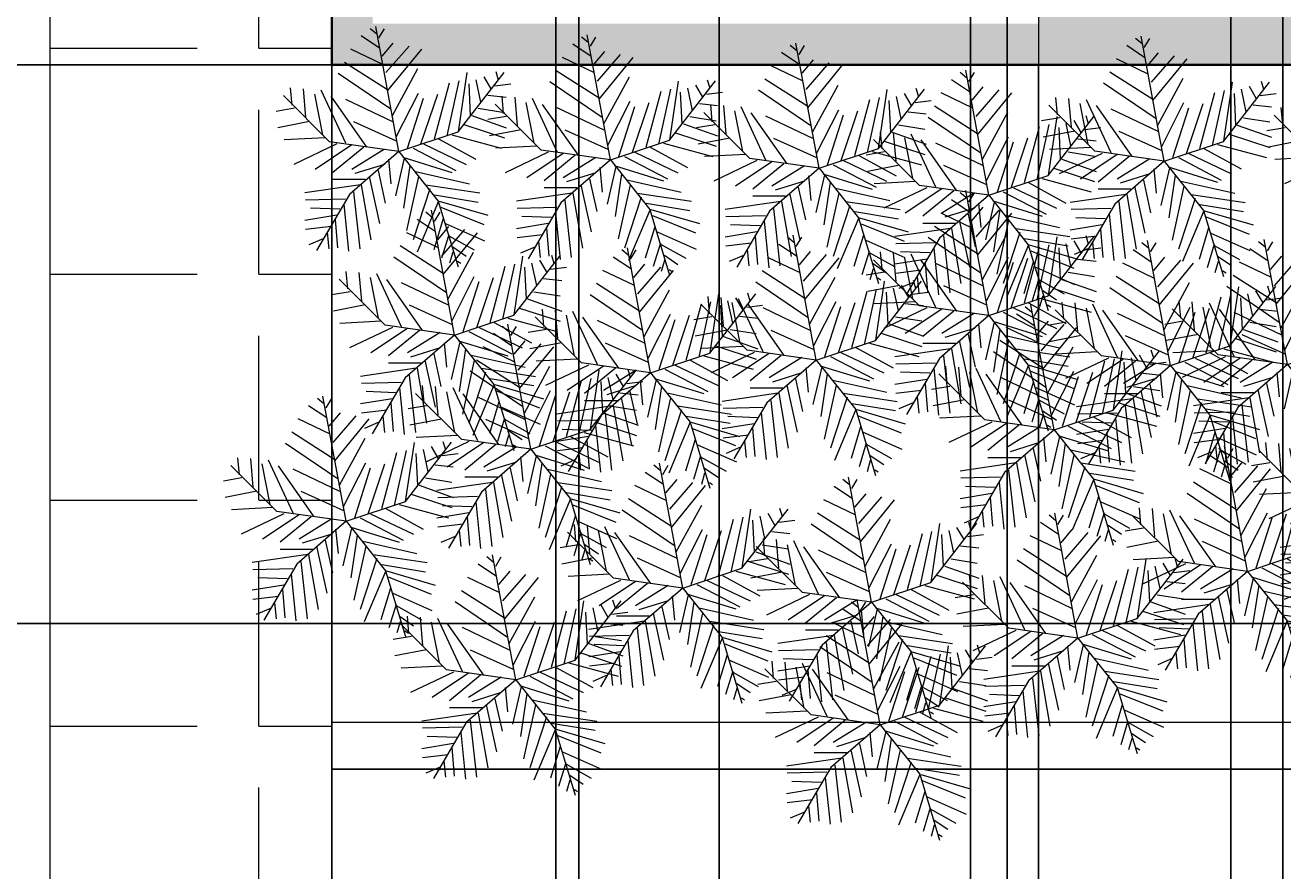
# Model space of a CAD drawing. Units: inches. Extents: x 818 to 1898, y 976 to 2364.
# Tile 20 of 96: x 1405 to 1512, y 1277 to 1349. Entities that reach past the tile are written whole.
import ezdxf

# ---------------------------------------------------------------- set-up
doc = ezdxf.new("R2010")
doc.units = ezdxf.units.IN
doc.header["$LTSCALE"] = 5
doc.header["$MEASUREMENT"] = 0
for name, color, linetype, lineweight in [('A-ANNO-DIMS', 2, 'Continuous', 18), ('A-GLAZ', 4, 'Continuous', 18), ('A-WALL', 7, 'Continuous', 40), ('C-PKNG', 8, 'Continuous', 18), ('C-PKNG-PATT', 9, 'Continuous', 9), ('L-PLNT-BEDS', 94, 'Continuous', 18)]:
    doc.layers.add(name, color=color, linetype=linetype, lineweight=lineweight)
for name, color, linetype, lineweight, true_color in [('A-GLAZ-PATT', 141, 'Continuous', 9, 0xadddf7), ('A-WALL-PATT', 251, 'Continuous', 13, 0x636466), ('L-PLNT', 116, 'Continuous', 13, 0x136734)]:
    doc.layers.add(name, color=color, linetype=linetype, lineweight=lineweight, true_color=true_color)
doc.styles.get("Standard").update_dxf_attribs({"font": 'arial.ttf'})
doc.dimstyles.get("Standard").update_dxf_attribs({"dimtxt": 0.18, "dimasz": 0.18, "dimexe": 0.18, "dimexo": 0.0625, "dimgap": 0.09, "dimtad": 0, "dimtih": 1, "dimtoh": 1, "dimdec": 4, "dimzin": 0, "dimdsep": 46, "dimtxsty": 'Standard', "dimcen": 0.09, "dimadec": 0, "dimazin": 0, "dimtfac": 1, "dimtdec": 4, "dimtofl": 0, "dimtmove": 0, "dimatfit": 3, "dimfxl": 1, "dimtolj": 1, "dimtzin": 0, "dimarcsym": 0})
pattern_1 = [(0, (0, 0), (0, 19.25), [14, -5.25]), (90, (0, 0), (-19.25, 1e-15), [14, -5.25])]

# ---------------------------------------------------------------- blocks, each defined once
blk = doc.blocks.new('SHRUB-ACCENT')
for p, q in [((10.44, 9.82), (8.47, 20.47)), ((8.8, 18.63), (7.25, 19.67)), ((8.53, 19.84), (7.99, 20.28)), ((8.74, 19.5), (9.21, 20.28)), ((9.08, 17.24), (6.37, 18.54)), ((9.01, 17.93), (9.96, 19.06)), ((9.35, 16.54), (11.31, 18.8)), ((9.48, 14.98), (12.39, 18.54)), ((9.48, 15.07), (5.82, 17.41)), ((9.75, 13.42), (5.28, 16.46)), ((9.89, 12.9), (12.06, 16.89)), ((15.49, 11.5), (19.41, 16.55)), ((15.51, 11.51), (16.25, 16.54)), ((17.68, 16.2), (18.29, 15.16)), ((18.69, 16.63), (18.9, 15.94)), ((1.35, 13.77), (1.22, 15.24)), ((2.3, 15.16), (2.51, 12.72)), ((3.79, 15.07), (5.89, 10.55)), ((13.48, 10.9), (14.76, 15.68)), ((14.56, 11.16), (15.58, 15.85)), ((16.39, 15.59), (16.53, 12.9)), ((17, 15.94), (17.41, 14.03)), ((18.62, 15.42), (19.98, 15.59)), ((4.55, 10.66), (0.62, 14.58)), ((3.25, 14.72), (3.93, 11.25)), ((7.72, 10.21), (4.67, 14.55)), ((5.89, 14.29), (9.89, 12.38)), ((10.23, 11.07), (12.12, 14.81)), ((11.17, 10.12), (12.53, 14.37)), ((12.33, 10.47), (13.75, 14.72)), ((18.02, 14.63), (19.57, 14.46)), ((1.56, 13.51), (0, 13.25)), ((16.66, 12.9), (19.57, 11.86)), ((17.2, 13.51), (19.44, 13.16)), ((2.84, 12.38), (0.14, 11.86)), ((6.57, 12.38), (10.23, 10.73)), ((15.98, 12.12), (19.44, 10.99)), ((4.2, 10.99), (0.68, 10.81)), ((10.44, 9.82), (15.49, 11.5)), ((13.82, 10.9), (17, 9.16)), ((14.97, 11.25), (19.17, 10.12)), ((5.15, 10.47), (1.49, 8.73)), ((6.43, 10.38), (3.32, 8.3)), ((10.44, 9.82), (4.55, 10.66)), ((7.45, 10.21), (4.81, 8.04)), ((10.44, 9.82), (6.23, 6.17)), ((9.21, 10.03), (6.43, 8.3)), ((10.44, 9.82), (13.8, 5.61)), ((11.65, 10.12), (15.31, 8.21)), ((12.53, 10.47), (16.19, 8.73)), ((9.21, 8.73), (6.7, 7.95)), ((9.55, 9.16), (9.75, 7.08)), ((10.9, 9.25), (10.16, 6.04)), ((10.77, 9.34), (14.97, 8.04)), ((11.38, 8.64), (10.84, 5)), ((7.92, 7.69), (8.8, 3.69)), ((8.67, 8.21), (9.28, 5.43)), ((12.12, 7.69), (11.11, 3.09)), ((11.85, 8.12), (16.46, 7.08)), ((7.18, 6.99), (2.44, 6.3)), ((7.59, 7.43), (4.81, 7.43)), ((7.25, 6.99), (8.06, 2.31)), ((13.07, 6.65), (11.65, 2.31)), ((12.73, 6.99), (17.34, 6.3)), ((5.89, 5.78), (2.51, 5.69)), ((6.23, 6.17), (3.43, 1.4)), ((6.57, 6.39), (7.11, 1.52)), ((13.82, 5.6), (11.99, 1.26)), ((13.48, 6.13), (17.2, 5.52)), ((13.8, 5.61), (15.49, 0)), ((13.88, 5.6), (18.02, 4.39)), ((5.15, 4.39), (2.44, 3.95)), ((5.42, 4.91), (2.91, 5)), ((5.76, 5.34), (6.16, 1.35)), ((14.02, 5.08), (17.68, 3.61)), ((4.67, 3.43), (2.51, 3.17)), ((5.01, 4.04), (5.21, 1.61)), ((14.22, 4.13), (13.41, 1.44)), ((14.43, 3.69), (17.74, 2.22)), ((4, 2.39), (2.78, 1.87)), ((4.33, 2.91), (4.47, 1.52)), ((14.7, 2.74), (14.09, 0.74)), ((14.7, 2.65), (16.86, 1.44)), ((15.04, 1.26), (14.76, 0.31)), ((15.04, 1.7), (16.19, 0.92)), ((15.44, 0.48), (15.71, 0.31))]:
    blk.add_line(p, q)
blk = doc.blocks.new('*D61')
at = {"layer": 'A-ANNO-DIMS', "color": 0, "lineweight": -2, "ltscale": 5, "transparency": 16777216}
for p, q in [((1071.73, 1203.03), (1071.73, 2363.87)), ((1430.73, 1203.03), (1430.73, 2363.87)), ((1071.91, 2363.69), (1250.94, 2363.69)), ((1430.55, 2363.69), (1251.51, 2363.69))]:
    blk.add_line(p, q, dxfattribs=at)
at = {"layer": 'A-ANNO-DIMS', "color": 0, "ltscale": 5, "transparency": 16777216}
for points in [[(1071.91, 2363.72), (1071.91, 2363.66), (1071.73, 2363.69)], [(1430.55, 2363.72), (1430.55, 2363.66), (1430.73, 2363.69)]]:
    blk.add_solid(points, dxfattribs=at)
at = {"layer": 'Defpoints', "color": 0, "ltscale": 5, "transparency": 16777216}
for p in [(1430.73, 2363.69), (1071.73, 1202.96), (1430.73, 1202.96)]:
    blk.add_point(p, dxfattribs=at)
at = {"layer": 'A-ANNO-DIMS', "color": 0, "ltscale": 5, "transparency": 16777216, "insert": (1251.23, 2363.69), "char_height": 0.18, "attachment_point": 5}
blk.add_mtext('\\A1;359', dxfattribs=at)
blk = doc.blocks.new('*D65')
at = {"layer": 'A-ANNO-DIMS', "color": 0, "lineweight": -2, "ltscale": 5, "transparency": 16777216}
for p, q in [((1430.73, 1346.02), (1430.73, 975.66)), ((1714.73, 1346.02), (1714.73, 975.66)), ((1430.91, 975.84), (1572.44, 975.84)), ((1714.55, 975.84), (1573.02, 975.84))]:
    blk.add_line(p, q, dxfattribs=at)
at = {"layer": 'A-ANNO-DIMS', "color": 0, "ltscale": 5, "transparency": 16777216}
for points in [[(1430.91, 975.87), (1430.91, 975.81), (1430.73, 975.84)], [(1714.55, 975.87), (1714.55, 975.81), (1714.73, 975.84)]]:
    blk.add_solid(points, dxfattribs=at)
at = {"layer": 'Defpoints', "color": 0, "ltscale": 5, "transparency": 16777216}
for p in [(1430.73, 1346.08), (1714.73, 1346.08), (1714.73, 975.84)]:
    blk.add_point(p, dxfattribs=at)
at = {"layer": 'A-ANNO-DIMS', "color": 0, "ltscale": 5, "transparency": 16777216, "insert": (1572.73, 975.84), "char_height": 0.18, "attachment_point": 5}
blk.add_mtext('\\A1;284', dxfattribs=at)
blk = doc.blocks.new('*D99')
at = {"layer": 'A-ANNO-DIMS', "color": 0, "lineweight": -2, "ltscale": 5, "transparency": 16777216}
for p, q in [((1391.88, 1071.12), (1391.88, 2363.87)), ((1449.82, 1071.12), (1449.82, 2363.87)), ((1392.06, 2363.69), (1420.45, 2363.69)), ((1449.64, 2363.69), (1421.24, 2363.69))]:
    blk.add_line(p, q, dxfattribs=at)
at = {"layer": 'A-ANNO-DIMS', "color": 0, "ltscale": 5, "transparency": 16777216}
for points in [[(1392.06, 2363.72), (1392.06, 2363.66), (1391.88, 2363.69)], [(1449.64, 2363.72), (1449.64, 2363.66), (1449.82, 2363.69)]]:
    blk.add_solid(points, dxfattribs=at)
at = {"layer": 'Defpoints', "color": 0, "ltscale": 5, "transparency": 16777216}
for p in [(1449.82, 2363.69), (1391.88, 1071.06), (1449.82, 1071.06)]:
    blk.add_point(p, dxfattribs=at)
at = {"layer": 'A-ANNO-DIMS', "color": 0, "ltscale": 5, "transparency": 16777216, "insert": (1420.85, 2363.69), "char_height": 0.18, "attachment_point": 5}
blk.add_mtext('\\A1;57.94', dxfattribs=at)
blk = doc.blocks.new('*D100')
at = {"layer": 'A-ANNO-DIMS', "color": 0, "lineweight": -2, "ltscale": 5, "transparency": 16777216}
for p, q in [((1449.82, 1071.12), (1449.82, 2363.87)), ((1507.3, 1071.12), (1507.3, 2363.87)), ((1450, 2363.69), (1478.17, 2363.69)), ((1507.12, 2363.69), (1478.95, 2363.69))]:
    blk.add_line(p, q, dxfattribs=at)
at = {"layer": 'A-ANNO-DIMS', "color": 0, "ltscale": 5, "transparency": 16777216}
for points in [[(1450, 2363.72), (1450, 2363.66), (1449.82, 2363.69)], [(1507.12, 2363.72), (1507.12, 2363.66), (1507.3, 2363.69)]]:
    blk.add_solid(points, dxfattribs=at)
at = {"layer": 'Defpoints', "color": 0, "ltscale": 5, "transparency": 16777216}
for p in [(1507.3, 2363.69), (1449.82, 1071.06), (1507.3, 1071.06)]:
    blk.add_point(p, dxfattribs=at)
at = {"layer": 'A-ANNO-DIMS', "color": 0, "ltscale": 5, "transparency": 16777216, "insert": (1478.56, 2363.69), "char_height": 0.18, "attachment_point": 5}
blk.add_mtext('\\A1;57.48', dxfattribs=at)
blk = doc.blocks.new('*D101')
at = {"layer": 'A-ANNO-DIMS', "color": 0, "lineweight": -2, "ltscale": 5, "transparency": 16777216}
for p, q in [((1507.3, 1071.12), (1507.3, 2363.87)), ((1565.48, 1071.12), (1565.48, 2363.87)), ((1507.48, 2363.69), (1536, 2363.69)), ((1565.3, 2363.69), (1536.78, 2363.69))]:
    blk.add_line(p, q, dxfattribs=at)
at = {"layer": 'A-ANNO-DIMS', "color": 0, "ltscale": 5, "transparency": 16777216}
for points in [[(1507.48, 2363.72), (1507.48, 2363.66), (1507.3, 2363.69)], [(1565.3, 2363.72), (1565.3, 2363.66), (1565.48, 2363.69)]]:
    blk.add_solid(points, dxfattribs=at)
at = {"layer": 'Defpoints', "color": 0, "ltscale": 5, "transparency": 16777216}
for p in [(1565.48, 2363.69), (1507.3, 1071.06), (1565.48, 1071.06)]:
    blk.add_point(p, dxfattribs=at)
at = {"layer": 'A-ANNO-DIMS', "color": 0, "ltscale": 5, "transparency": 16777216, "insert": (1536.39, 2363.69), "char_height": 0.18, "attachment_point": 5}
blk.add_mtext('\\A1;58.19', dxfattribs=at)
blk = doc.blocks.new('*D113')
at = {"layer": 'A-ANNO-DIMS', "color": 0, "lineweight": -2, "ltscale": 5, "transparency": 16777216}
for p, q in [((1430.79, 1346.08), (1897.92, 1346.08)), ((1897.74, 1345.9), (1897.74, 1316.26)), ((1897.74, 1286.26), (1897.74, 1315.9)), ((1430.79, 1286.08), (1897.92, 1286.08))]:
    blk.add_line(p, q, dxfattribs=at)
at = {"layer": 'A-ANNO-DIMS', "color": 0, "ltscale": 5, "transparency": 16777216}
for points in [[(1897.71, 1345.9), (1897.77, 1345.9), (1897.74, 1346.08)], [(1897.71, 1286.26), (1897.77, 1286.26), (1897.74, 1286.08)]]:
    blk.add_solid(points, dxfattribs=at)
at = {"layer": 'Defpoints', "color": 0, "ltscale": 5, "transparency": 16777216}
for p in [(1430.73, 1346.08), (1897.74, 1346.08), (1430.73, 1286.08)]:
    blk.add_point(p, dxfattribs=at)
at = {"layer": 'A-ANNO-DIMS', "color": 0, "ltscale": 5, "transparency": 16777216, "insert": (1897.74, 1316.08), "char_height": 0.18, "attachment_point": 5}
blk.add_mtext('\\A1;60', dxfattribs=at)
blk = doc.blocks.new('*D115')
at = {"layer": 'A-ANNO-DIMS', "color": 0, "lineweight": -2, "ltscale": 5, "transparency": 16777216}
for p, q in [((1766.29, 1377.66), (818.03, 1377.66)), ((818.21, 1377.48), (818.21, 1338.26)), ((818.21, 1298.68), (818.21, 1337.9)), ((1766.29, 1298.5), (818.03, 1298.5))]:
    blk.add_line(p, q, dxfattribs=at)
at = {"layer": 'A-ANNO-DIMS', "color": 0, "ltscale": 5, "transparency": 16777216}
for points in [[(818.18, 1377.48), (818.24, 1377.48), (818.21, 1377.66)], [(818.18, 1298.68), (818.24, 1298.68), (818.21, 1298.5)]]:
    blk.add_solid(points, dxfattribs=at)
at = {"layer": 'Defpoints', "color": 0, "ltscale": 5, "transparency": 16777216}
for p in [(818.21, 1377.66), (1766.35, 1377.66), (1766.35, 1298.5)]:
    blk.add_point(p, dxfattribs=at)
at = {"layer": 'A-ANNO-DIMS', "color": 0, "ltscale": 5, "transparency": 16777216, "insert": (818.21, 1338.08), "char_height": 0.18, "attachment_point": 5}
blk.add_mtext('\\A1;79.15', dxfattribs=at)
blk = doc.blocks.new('*D159')
at = {"layer": 'A-ANNO-DIMS', "color": 0, "lineweight": -2, "ltscale": 5, "transparency": 16777216}
for p, q in [((1206.73, 1687.02), (1206.73, 975.66)), ((1463.73, 1687.02), (1463.73, 975.66)), ((1206.91, 975.84), (1334.93, 975.84)), ((1463.55, 975.84), (1335.52, 975.84))]:
    blk.add_line(p, q, dxfattribs=at)
at = {"layer": 'A-ANNO-DIMS', "color": 0, "ltscale": 5, "transparency": 16777216}
for points in [[(1206.91, 975.87), (1206.91, 975.81), (1206.73, 975.84)], [(1463.55, 975.87), (1463.55, 975.81), (1463.73, 975.84)]]:
    blk.add_solid(points, dxfattribs=at)
at = {"layer": 'Defpoints', "color": 0, "ltscale": 5, "transparency": 16777216}
for p in [(1206.73, 1687.08), (1463.73, 1687.08), (1463.73, 975.84)]:
    blk.add_point(p, dxfattribs=at)
at = {"layer": 'A-ANNO-DIMS', "color": 0, "ltscale": 5, "transparency": 16777216, "insert": (1335.23, 975.84), "char_height": 0.18, "attachment_point": 5}
blk.add_mtext('\\A1;257', dxfattribs=at)
blk = doc.blocks.new('*D160')
at = {"layer": 'A-ANNO-DIMS', "color": 0, "lineweight": -2, "ltscale": 5, "transparency": 16777216}
for p, q in [((1463.73, 1687.02), (1463.73, 975.66)), ((1511.73, 1687.02), (1511.73, 975.66)), ((1463.91, 975.84), (1487.5, 975.84)), ((1511.55, 975.84), (1487.95, 975.84))]:
    blk.add_line(p, q, dxfattribs=at)
at = {"layer": 'A-ANNO-DIMS', "color": 0, "ltscale": 5, "transparency": 16777216}
for points in [[(1463.91, 975.87), (1463.91, 975.81), (1463.73, 975.84)], [(1511.55, 975.87), (1511.55, 975.81), (1511.73, 975.84)]]:
    blk.add_solid(points, dxfattribs=at)
at = {"layer": 'Defpoints', "color": 0, "ltscale": 5, "transparency": 16777216}
for p in [(1463.73, 1687.08), (1511.73, 1687.08), (1511.73, 975.84)]:
    blk.add_point(p, dxfattribs=at)
at = {"layer": 'A-ANNO-DIMS', "color": 0, "ltscale": 5, "transparency": 16777216, "insert": (1487.73, 975.84), "char_height": 0.18, "attachment_point": 5}
blk.add_mtext('\\A1;48', dxfattribs=at)
blk = doc.blocks.new('*D167')
at = {"layer": 'A-ANNO-DIMS', "color": 0, "lineweight": -2, "ltscale": 5, "transparency": 16777216}
for p, q in [((1345.97, 1486.18), (1345.97, 975.66)), ((1430.73, 1486.18), (1430.73, 975.66)), ((1346.15, 975.84), (1387.95, 975.84)), ((1430.55, 975.84), (1388.74, 975.84))]:
    blk.add_line(p, q, dxfattribs=at)
at = {"layer": 'A-ANNO-DIMS', "color": 0, "ltscale": 5, "transparency": 16777216}
for points in [[(1346.15, 975.87), (1346.15, 975.81), (1345.97, 975.84)], [(1430.55, 975.87), (1430.55, 975.81), (1430.73, 975.84)]]:
    blk.add_solid(points, dxfattribs=at)
at = {"layer": 'Defpoints', "color": 0, "ltscale": 5, "transparency": 16777216}
for p in [(1345.97, 1486.24), (1430.73, 1486.24), (1430.73, 975.84)]:
    blk.add_point(p, dxfattribs=at)
at = {"layer": 'A-ANNO-DIMS', "color": 0, "ltscale": 5, "transparency": 16777216, "insert": (1388.35, 975.84), "char_height": 0.18, "attachment_point": 5}
blk.add_mtext('\\A1;84.76', dxfattribs=at)
blk = doc.blocks.new('*D182')
at = {"layer": 'A-ANNO-DIMS', "color": 0, "lineweight": -2, "ltscale": 5, "transparency": 16777216}
for p, q in [((1463.73, 1687.02), (1463.73, 975.66)), ((1559.73, 1687.02), (1559.73, 975.66)), ((1463.91, 975.84), (1511.51, 975.84)), ((1559.55, 975.84), (1511.94, 975.84))]:
    blk.add_line(p, q, dxfattribs=at)
at = {"layer": 'A-ANNO-DIMS', "color": 0, "ltscale": 5, "transparency": 16777216}
for points in [[(1463.91, 975.87), (1463.91, 975.81), (1463.73, 975.84)], [(1559.55, 975.87), (1559.55, 975.81), (1559.73, 975.84)]]:
    blk.add_solid(points, dxfattribs=at)
at = {"layer": 'Defpoints', "color": 0, "ltscale": 5, "transparency": 16777216}
for p in [(1463.73, 1687.08), (1559.73, 1687.08), (1559.73, 975.84)]:
    blk.add_point(p, dxfattribs=at)
at = {"layer": 'A-ANNO-DIMS', "color": 0, "ltscale": 5, "transparency": 16777216, "insert": (1511.73, 975.84), "char_height": 0.18, "attachment_point": 5}
blk.add_mtext('\\A1;96', dxfattribs=at)
blk = doc.blocks.new('*D189')
at = {"layer": 'A-ANNO-DIMS', "color": 0, "lineweight": -2, "ltscale": 5, "transparency": 16777216}
for p, q in [((1430.73, 1346.02), (1430.73, 975.66)), ((1490.92, 1346.02), (1490.92, 975.66)), ((1430.91, 975.84), (1460.43, 975.84)), ((1490.74, 975.84), (1461.22, 975.84))]:
    blk.add_line(p, q, dxfattribs=at)
at = {"layer": 'A-ANNO-DIMS', "color": 0, "ltscale": 5, "transparency": 16777216}
for points in [[(1430.91, 975.87), (1430.91, 975.81), (1430.73, 975.84)], [(1490.74, 975.87), (1490.74, 975.81), (1490.92, 975.84)]]:
    blk.add_solid(points, dxfattribs=at)
at = {"layer": 'Defpoints', "color": 0, "ltscale": 5, "transparency": 16777216}
for p in [(1430.73, 1346.08), (1490.92, 1346.08), (1490.92, 975.84)]:
    blk.add_point(p, dxfattribs=at)
at = {"layer": 'A-ANNO-DIMS', "color": 0, "ltscale": 5, "transparency": 16777216, "insert": (1460.82, 975.84), "char_height": 0.18, "attachment_point": 5}
blk.add_mtext('\\A1;60.19', dxfattribs=at)
blk = doc.blocks.new('*D190')
at = {"layer": 'A-ANNO-DIMS', "color": 0, "lineweight": -2, "ltscale": 5, "transparency": 16777216}
for p, q in [((1430.66, 1409.05), (818.03, 1409.05)), ((818.21, 1408.87), (818.21, 1377.75)), ((818.21, 1346.26), (818.21, 1377.38)), ((1430.66, 1346.08), (818.03, 1346.08))]:
    blk.add_line(p, q, dxfattribs=at)
at = {"layer": 'A-ANNO-DIMS', "color": 0, "ltscale": 5, "transparency": 16777216}
for points in [[(818.18, 1408.87), (818.24, 1408.87), (818.21, 1409.05)], [(818.18, 1346.26), (818.24, 1346.26), (818.21, 1346.08)]]:
    blk.add_solid(points, dxfattribs=at)
at = {"layer": 'Defpoints', "color": 0, "ltscale": 5, "transparency": 16777216}
for p in [(818.21, 1409.05), (1430.73, 1409.05), (1430.73, 1346.08)]:
    blk.add_point(p, dxfattribs=at)
at = {"layer": 'A-ANNO-DIMS', "color": 0, "ltscale": 5, "transparency": 16777216, "insert": (818.21, 1377.57), "char_height": 0.18, "attachment_point": 5}
blk.add_mtext('\\A1;62.97', dxfattribs=at)
blk = doc.blocks.new('*D198')
at = {"layer": 'A-ANNO-DIMS', "color": 0, "lineweight": -2, "ltscale": 5, "transparency": 16777216}
for p, q in [((1741.84, 1545.02), (1741.84, 975.66)), ((1430.73, 1346.02), (1430.73, 975.66)), ((1430.91, 975.84), (1585.91, 975.84)), ((1741.66, 975.84), (1586.66, 975.84))]:
    blk.add_line(p, q, dxfattribs=at)
at = {"layer": 'A-ANNO-DIMS', "color": 0, "ltscale": 5, "transparency": 16777216}
for points in [[(1430.91, 975.87), (1430.91, 975.81), (1430.73, 975.84)], [(1741.66, 975.87), (1741.66, 975.81), (1741.84, 975.84)]]:
    blk.add_solid(points, dxfattribs=at)
at = {"layer": 'Defpoints', "color": 0, "ltscale": 5, "transparency": 16777216}
for p in [(1741.84, 1545.08), (1430.73, 1346.08), (1741.84, 975.84)]:
    blk.add_point(p, dxfattribs=at)
at = {"layer": 'A-ANNO-DIMS', "color": 0, "ltscale": 5, "transparency": 16777216, "insert": (1586.28, 975.84), "char_height": 0.18, "attachment_point": 5}
blk.add_mtext('\\A1;311.1', dxfattribs=at)
blk = doc.blocks.new('*D214')
at = {"layer": 'A-ANNO-DIMS', "color": 0, "lineweight": -2, "ltscale": 5, "transparency": 16777216}
for p, q in [((1511.73, 1687.02), (1511.73, 975.66)), ((1714.73, 1687.02), (1714.73, 975.66)), ((1511.91, 975.84), (1612.93, 975.84)), ((1714.55, 975.84), (1613.52, 975.84))]:
    blk.add_line(p, q, dxfattribs=at)
at = {"layer": 'A-ANNO-DIMS', "color": 0, "ltscale": 5, "transparency": 16777216}
for points in [[(1511.91, 975.87), (1511.91, 975.81), (1511.73, 975.84)], [(1714.55, 975.87), (1714.55, 975.81), (1714.73, 975.84)]]:
    blk.add_solid(points, dxfattribs=at)
at = {"layer": 'Defpoints', "color": 0, "ltscale": 5, "transparency": 16777216}
for p in [(1511.73, 1687.08), (1714.73, 1687.08), (1714.73, 975.84)]:
    blk.add_point(p, dxfattribs=at)
at = {"layer": 'A-ANNO-DIMS', "color": 0, "ltscale": 5, "transparency": 16777216, "insert": (1613.23, 975.84), "char_height": 0.18, "attachment_point": 5}
blk.add_mtext('\\A1;203', dxfattribs=at)
blk = doc.blocks.new('*D242')
at = {"layer": 'A-ANNO-DIMS', "color": 0, "lineweight": -2, "ltscale": 5, "transparency": 16777216}
for p, q in [((1488.26, 1948.6), (1488.26, 975.66)), ((1513.23, 1948.6), (1513.23, 975.66)), ((1488.44, 975.84), (1500.35, 975.84)), ((1513.05, 975.84), (1501.14, 975.84))]:
    blk.add_line(p, q, dxfattribs=at)
at = {"layer": 'A-ANNO-DIMS', "color": 0, "ltscale": 5, "transparency": 16777216}
for points in [[(1488.44, 975.87), (1488.44, 975.81), (1488.26, 975.84)], [(1513.05, 975.87), (1513.05, 975.81), (1513.23, 975.84)]]:
    blk.add_solid(points, dxfattribs=at)
at = {"layer": 'Defpoints', "color": 0, "ltscale": 5, "transparency": 16777216}
for p in [(1488.26, 1948.66), (1513.23, 1948.66), (1513.23, 975.84)]:
    blk.add_point(p, dxfattribs=at)
at = {"layer": 'A-ANNO-DIMS', "color": 0, "ltscale": 5, "transparency": 16777216, "insert": (1500.74, 975.84), "char_height": 0.18, "attachment_point": 5}
blk.add_mtext('\\A1;24.97', dxfattribs=at)
blk = doc.blocks.new('*D243')
at = {"layer": 'A-ANNO-DIMS', "color": 0, "lineweight": -2, "ltscale": 5, "transparency": 16777216}
for p, q in [((1451.77, 2020.02), (1451.77, 975.66)), ((1590.73, 2020.02), (1590.73, 975.66)), ((1451.95, 975.84), (1520.79, 975.84)), ((1590.55, 975.84), (1521.7, 975.84))]:
    blk.add_line(p, q, dxfattribs=at)
at = {"layer": 'A-ANNO-DIMS', "color": 0, "ltscale": 5, "transparency": 16777216}
for points in [[(1451.95, 975.87), (1451.95, 975.81), (1451.77, 975.84)], [(1590.55, 975.87), (1590.55, 975.81), (1590.73, 975.84)]]:
    blk.add_solid(points, dxfattribs=at)
at = {"layer": 'Defpoints', "color": 0, "ltscale": 5, "transparency": 16777216}
for p in [(1451.77, 2020.08), (1590.73, 2020.08), (1590.73, 975.84)]:
    blk.add_point(p, dxfattribs=at)
at = {"layer": 'A-ANNO-DIMS', "color": 0, "ltscale": 5, "transparency": 16777216, "insert": (1521.25, 975.84), "char_height": 0.18, "attachment_point": 5}
blk.add_mtext('\\A1;138.96', dxfattribs=at)
blk = doc.blocks.new('*D253')
at = {"layer": 'A-ANNO-DIMS', "color": 0, "lineweight": -2, "ltscale": 5, "transparency": 16777216}
for p, q in [((1485.12, 2053.02), (1485.12, 975.66)), ((1538.52, 2053.02), (1538.52, 975.66)), ((1485.3, 975.84), (1511.42, 975.84)), ((1538.34, 975.84), (1512.21, 975.84))]:
    blk.add_line(p, q, dxfattribs=at)
at = {"layer": 'A-ANNO-DIMS', "color": 0, "ltscale": 5, "transparency": 16777216}
for points in [[(1485.3, 975.87), (1485.3, 975.81), (1485.12, 975.84)], [(1538.34, 975.87), (1538.34, 975.81), (1538.52, 975.84)]]:
    blk.add_solid(points, dxfattribs=at)
at = {"layer": 'Defpoints', "color": 0, "ltscale": 5, "transparency": 16777216}
for p in [(1485.12, 2053.08), (1538.52, 2053.08), (1538.52, 975.84)]:
    blk.add_point(p, dxfattribs=at)
at = {"layer": 'A-ANNO-DIMS', "color": 0, "ltscale": 5, "transparency": 16777216, "insert": (1511.82, 975.84), "char_height": 0.18, "attachment_point": 5}
blk.add_mtext('\\A1;53.39', dxfattribs=at)

msp = doc.modelspace()

# ---------------------------------------------------------------- hatches: boundary and pattern name
at = {"layer": 'A-GLAZ-PATT', "ltscale": 5}
h = msp.add_hatch(color=256, dxfattribs=at)
h.dxf.hatch_style = 1
h.paths.add_polyline_path([(1283.8183, 1504.5782), (1206.7251, 1504.5782), (1206.7251, 1501.0782), (1283.8183, 1501.0782)])
h.paths.add_polyline_path([(1283.8183, 1510.0782), (1206.7251, 1510.0782), (1206.7251, 1506.5782), (1283.8183, 1506.5782)])
h.paths.add_polyline_path([(1490.9163, 1355.0782), (1439.7252, 1355.0782), (1439.7252, 1409.0522), (1436.2252, 1409.0522), (1436.2252, 1351.5782), (1490.9163, 1351.5782)])
h.paths.add_polyline_path([(1434.2252, 1409.0522), (1430.7251, 1409.0522), (1430.7251, 1346.0782), (1435.0799, 1346.0782), (1435.0731, 1346.1152), (1435.1501, 1346.0782), (1490.9163, 1346.0782), (1490.9163, 1349.5782), (1434.2252, 1349.5782)])
h.paths.add_polyline_path([(1714.7251, 1545.0782), (1711.2252, 1545.0782), (1711.2252, 1521.0782), (1714.7251, 1521.0782)])
h.paths.add_polyline_path([(1709.2252, 1545.0782), (1705.7252, 1545.0782), (1705.7252, 1521.0782), (1709.2252, 1521.0782)])
h.paths.add_polyline_path([(1714.7251, 1687.0782), (1711.2252, 1687.0782), (1711.2252, 1649.9029), (1714.7251, 1649.9029)])
h.paths.add_polyline_path([(1709.2252, 1687.0782), (1705.7252, 1687.0782), (1705.7252, 1649.9029), (1709.2252, 1649.9029)])
h.paths.add_polyline_path([(1709.2252, 1745.5584), (1705.7252, 1745.5584), (1705.7252, 1717.3178), (1709.2252, 1717.3178)])
h.paths.add_polyline_path([(1714.7251, 1745.5584), (1711.2252, 1745.5584), (1711.2252, 1717.3178), (1714.7251, 1717.3178)])
h.paths.add_polyline_path([(1714.7251, 2014.5114), (1711.2252, 2014.5114), (1711.2252, 1962.0338), (1714.7251, 1962.0338)])
h.paths.add_polyline_path([(1709.2252, 2014.5114), (1705.7252, 2014.5114), (1705.7252, 1962.0338), (1709.2252, 1962.0338)])
h.paths.add_polyline_path([(1538.5155, 2047.5782), (1485.1216, 2047.5782), (1485.1216, 2044.0782), (1538.5155, 2044.0782)])
h.paths.add_polyline_path([(1538.5155, 2053.0782), (1485.1216, 2053.0782), (1485.1216, 2049.5782), (1538.5155, 2049.5782)])
h.paths.add_polyline_path([(1388.0315, 2047.5782), (1330.305, 2047.5782), (1330.305, 2044.0782), (1388.0315, 2044.0782)])
h.paths.add_polyline_path([(1388.0315, 2053.0782), (1330.305, 2053.0782), (1330.305, 2049.5782), (1388.0315, 2049.5782)])
h.paths.add_polyline_path([(1262.2252, 2019.2871), (1258.7252, 2019.2871), (1258.7252, 1928.9218), (1262.2252, 1928.9218)])
h.paths.add_polyline_path([(1267.7252, 2019.2871), (1264.2252, 2019.2871), (1264.2252, 1928.9218), (1267.7252, 1928.9218)])
h.paths.add_polyline_path([(1262.2252, 1862.9652), (1258.7252, 1862.9652), (1258.7252, 1814.9652), (1262.2252, 1814.9652)])
h.paths.add_polyline_path([(1267.7252, 1862.9652), (1264.2252, 1862.9652), (1264.2252, 1814.9652), (1267.7252, 1814.9652)])
h.paths.add_polyline_path([(1262.2252, 1755.3321), (1258.7252, 1755.3321), (1258.7252, 1707.3321), (1262.2252, 1707.3321)])
h.paths.add_polyline_path([(1267.7252, 1755.3321), (1264.2252, 1755.3321), (1264.2252, 1707.3321), (1267.7252, 1707.3321)])
h.paths.add_polyline_path([(1251.9333, 1692.5782), (1206.7251, 1692.5782), (1206.7251, 1687.0782), (1251.9333, 1687.0782)])
h.paths.add_polyline_path([(1251.9333, 1700.0782), (1206.7251, 1700.0782), (1206.7251, 1694.5782), (1251.9333, 1694.5782)])
at = {"layer": 'A-WALL-PATT', "ltscale": 5}
h = msp.add_hatch(color=256, dxfattribs=at)
h.dxf.hatch_style = 1
h.paths.add_polyline_path([(1714.7251, 1521.0782), (1705.7252, 1521.0782), (1705.7252, 1467.0782), (1654.7252, 1467.0782), (1654.7252, 1463.0782), (1705.7252, 1463.0782), (1705.7252, 1355.0782), (1622.7252, 1355.0782), (1622.7252, 1379.0782), (1622.7252, 1386.6857), (1616.7252, 1386.6857), (1616.7252, 1355.0782), (1490.9163, 1355.0782), (1490.9163, 1346.0782), (1544.7605, 1346.0782), (1544.6132, 1346.8783), (1544.6729, 1346.84), (1544.6299, 1346.7874), (1544.7605, 1346.0782), (1555.1299, 1346.0782), (1555.1299, 1341.5528), (1556.1599, 1340.8639), (1556.5281, 1338.8654), (1660.3141, 1338.8654), (1660.3141, 1346.0782), (1705.7252, 1346.0782), (1705.7252, 1345.0768), (1705.8704, 1344.58), (1705.7252, 1344.3933), (1705.7252, 1334.9904), (1705.8704, 1334.4936), (1705.7252, 1334.3068), (1705.7252, 1316.2253), (1707.3573, 1316.7694), (1707.3847, 1316.8046), (1707.3807, 1316.7771), (1705.7252, 1316.2253), (1705.7252, 1314.1392), (1705.7252, 1312.0957), (1705.8703, 1312.0739), (1705.7252, 1311.8873), (1705.7252, 1310.7121), (1706.5603, 1307.9282), (1707.8887, 1307.1831), (1714.7251, 1307.1831), (1714.7251, 1346.0782)])
at = {"layer": 'C-PKNG-PATT', "ltscale": 5}
h = msp.add_hatch(dxfattribs=at)
h.set_pattern_fill('ANGLE', color=256, scale=70)
h.set_pattern_definition(pattern_1)
h.paths.add_polyline_path([(1430.7251, 1211.9642), (1430.7251, 1486.2383), (1406.7252, 1486.2383), (1406.7252, 1235.9642), (1116.1882, 1235.9642), (1116.1882, 1485.2035), (1345.9651, 1485.2035), (1345.9651, 1501.0782), (1206.7251, 1501.0782), (1197.7252, 1501.0782), (1083.7252, 1501.0782), (1083.7252, 1485.2035), (1083.7252, 1211.9642)])
h = msp.add_hatch(dxfattribs=at)
h.set_pattern_fill('ANGLE', color=256, scale=70)
h.set_pattern_definition(pattern_1)
h.paths.add_polyline_path([(1116.1882, 1485.2035), (1345.9651, 1485.2035), (1345.9651, 1501.0782), (1206.7251, 1501.0782), (1197.7252, 1501.0782), (1083.7252, 1501.0782), (1083.7252, 1485.2035), (1083.7252, 1211.9642), (1430.7251, 1211.9642), (1430.7251, 1271.1621), (1430.7251, 1290.0782), (1430.7251, 1346.0782), (1430.7251, 1486.2383), (1406.7252, 1486.2383), (1406.7252, 1235.9642), (1116.1882, 1235.9642)])

# ---------------------------------------------------------------- linework, layer by layer
at = {"layer": 'A-GLAZ'}
msp.add_line((1490.9163, 1355.0782), (1490.9163, 1346.0782), dxfattribs=at)
at = {"layer": 'A-WALL'}
for p, q in [((1430.7251, 1501.0782), (1430.7251, 1346.0782)), ((1430.7251, 1346.0782), (1555.1299, 1346.0782))]:
    msp.add_line(p, q, dxfattribs=at)
at = {"layer": 'C-PKNG'}
for p, q in [((1406.7252, 1486.2383), (1406.7252, 1235.9642)), ((1430.7251, 1290.0782), (1430.7251, 1271.1621))]:
    msp.add_line(p, q, dxfattribs=at)
at = {"layer": 'C-PKNG', "ltscale": 5}
msp.add_line((1430.7251, 1346.0782), (1430.7251, 1290.0782), dxfattribs=at)
at = {"layer": 'L-PLNT'}
for p, q in [((1434.8076, 1347.5019), (1433.2499, 1348.5438)), ((1434.5367, 1348.7175), (1433.9949, 1349.1516)), ((1436.4411, 1338.6891), (1434.478, 1349.3457)), ((1434.7399, 1348.3701), (1435.2141, 1349.1516)), ((1435.0785, 1346.1126), (1432.3695, 1347.415)), ((1435.0108, 1346.8074), (1435.9591, 1347.936)), ((1435.3494, 1345.4181), (1437.3136, 1347.6756)), ((1435.485, 1343.8551), (1438.3972, 1347.415)), ((1435.7559, 1342.2923), (1431.2859, 1345.3311)), ((1435.485, 1343.9421), (1431.8277, 1346.2863)), ((1435.8912, 1341.7713), (1438.0586, 1345.7654)), ((1441.4889, 1340.3717), (1445.415, 1345.4196)), ((1441.5127, 1340.3822), (1442.2577, 1345.4181)), ((1444.6958, 1345.5048), (1444.8988, 1344.8103)), ((1439.4808, 1339.7744), (1440.7676, 1344.5498)), ((1440.5644, 1340.0348), (1441.5803, 1344.7235)), ((1442.393, 1344.4629), (1442.5286, 1341.7713)), ((1443.0025, 1344.8103), (1443.409, 1342.9001)), ((1443.6799, 1345.0707), (1444.2894, 1344.0288)), ((1444.6281, 1344.2892), (1445.9826, 1344.4629)), ((1430.5519, 1339.5304), (1426.6258, 1343.4565)), ((1427.3577, 1342.6397), (1427.2224, 1344.1157)), ((1428.306, 1344.0288), (1428.509, 1341.5978)), ((1429.2541, 1343.5947), (1429.9314, 1340.1218)), ((1429.7959, 1343.9421), (1431.8954, 1339.427)), ((1433.724, 1339.0798), (1430.6764, 1343.421)), ((1431.8954, 1343.1606), (1435.8912, 1341.2504)), ((1436.23, 1339.9481), (1438.1263, 1343.6816)), ((1437.1781, 1338.9929), (1438.5326, 1343.2473)), ((1438.3295, 1339.3403), (1439.7517, 1343.5947)), ((1444.0185, 1343.5079), (1445.5762, 1343.3343)), ((1427.561, 1342.3791), (1426.0032, 1342.1187)), ((1443.2058, 1342.3791), (1445.4406, 1342.0319)), ((1428.8478, 1341.2504), (1426.1388, 1340.7294)), ((1432.5727, 1341.2504), (1436.23, 1339.6007)), ((1441.9866, 1340.99), (1445.4406, 1339.8611)), ((1442.664, 1341.7713), (1445.5762, 1340.7294)), ((1436.4411, 1338.6891), (1441.4889, 1340.3717)), ((1440.9709, 1340.1218), (1445.1697, 1338.9929)), ((1430.2023, 1339.8611), (1426.6806, 1339.6875)), ((1431.1504, 1339.3403), (1427.4933, 1337.6038)), ((1432.4372, 1339.2533), (1429.3219, 1337.1695)), ((1436.4411, 1338.6891), (1430.5519, 1339.5304)), ((1433.4531, 1339.0798), (1430.8118, 1336.9091)), ((1435.2141, 1338.9062), (1432.4372, 1337.1695)), ((1437.6522, 1338.9929), (1441.3094, 1337.0828)), ((1438.5326, 1339.3403), (1442.1898, 1337.6038)), ((1439.8194, 1339.7744), (1443.0025, 1338.0379)), ((1436.4411, 1338.6891), (1432.2345, 1335.0434)), ((1435.5526, 1338.0379), (1435.7559, 1335.9541)), ((1436.9072, 1338.1247), (1436.1623, 1334.9122)), ((1436.4411, 1338.6891), (1439.8063, 1334.4826)), ((1436.7718, 1338.2114), (1440.9709, 1336.9091)), ((1435.2141, 1337.6038), (1432.7081, 1336.8223)), ((1434.6723, 1337.0828), (1435.2817, 1334.3044)), ((1437.3813, 1337.5169), (1436.8395, 1333.8703)), ((1437.8554, 1336.996), (1442.4607, 1335.9541)), ((1433.1822, 1335.8672), (1428.4413, 1335.1726)), ((1433.5887, 1336.3013), (1430.8118, 1336.3013)), ((1433.2499, 1335.8672), (1434.0628, 1331.1786)), ((1433.9272, 1336.5619), (1434.8076, 1332.5679)), ((1438.1263, 1336.5619), (1437.1104, 1331.9601)), ((1438.7358, 1335.8672), (1443.3411, 1335.1726)), ((1431.8954, 1334.6516), (1428.509, 1334.5648)), ((1432.2345, 1335.0434), (1429.4302, 1330.276)), ((1432.5727, 1335.2594), (1433.1145, 1330.3972)), ((1439.0744, 1335.52), (1437.6522, 1331.1786)), ((1439.4808, 1334.9989), (1443.2058, 1334.3911)), ((1431.4214, 1333.7833), (1428.9155, 1333.8703)), ((1431.76, 1334.2175), (1432.1663, 1330.2235)), ((1439.8194, 1334.4781), (1437.9908, 1330.1367)), ((1439.8063, 1334.4826), (1441.4889, 1328.8738)), ((1439.8873, 1334.4781), (1444.0185, 1333.2625)), ((1440.0226, 1333.957), (1443.6799, 1332.481)), ((1431.1504, 1333.2625), (1428.4413, 1332.8284)), ((1431.015, 1332.9151), (1431.2182, 1330.4841)), ((1440.2258, 1333.002), (1439.4131, 1330.3104)), ((1440.4291, 1332.5679), (1443.7476, 1331.0919)), ((1430.6764, 1332.3073), (1428.509, 1332.0469)), ((1430.3377, 1331.7864), (1430.4732, 1330.3972)), ((1440.7, 1331.6128), (1440.0903, 1329.6157)), ((1440.7, 1331.526), (1442.8672, 1330.3104)), ((1429.9991, 1331.2654), (1428.7799, 1330.7445)), ((1441.0385, 1330.5708), (1442.1898, 1329.7894)), ((1441.0385, 1330.1367), (1440.7676, 1329.1816)), ((1441.4448, 1329.3553), (1441.7157, 1329.1816))]:
    msp.add_line(p, q, dxfattribs=at)
at = {"layer": 'L-PLNT-BEDS', "ltscale": 5}
for points in [[(1430.7251, 1286.0782), (1701.3688, 1286.0782, 0.41421356), (1713.3688, 1298.0782), (1713.3688, 1307.1831)], [(1430.7251, 1290.0782), (1701.3688, 1290.0782, 0.41421356), (1709.3688, 1298.0782), (1709.3688, 1307.1831)]]:
    msp.add_lwpolyline(points, format="xyb", dxfattribs=at)

# ---------------------------------------------------------------- block references
at = {"layer": 'L-PLNT'}
for p in [(1444.0148, 1328.1632), (1491.1766, 1328.0566), (1461.7893, 1327.4528), (1510.3731, 1327.216), (1476.2459, 1325.1479), (1476.2459, 1314.9024), (1430.7431, 1313.2449), (1461.5523, 1311.1137), (1447.4457, 1310.0337), (1491.7184, 1310.6401), (1501.674, 1310.7268), (1481.7995, 1305.1779), (1437.2448, 1303.5203), (1509.055, 1298.6736), (1421.5143, 1297.3793), (1498.2864, 1293.1169), (1450.1766, 1291.6961), (1466.2671, 1290.4852), (1483.8298, 1287.4337), (1435.957, 1283.8817), (1467.0032, 1280.0457)]:
    msp.add_blockref('SHRUB-ACCENT', p, dxfattribs=at)

# ---------------------------------------------------------------- dimensions: what is measured, and where the dimension line sits
at = {"layer": 'A-ANNO-DIMS', "ltscale": 5}
for base, p1, p2, override, picture, middle in [((1430.7251, 2363.6929), (1071.7251, 1202.9642), (1430.7251, 1202.9642), {"dimdec": 0, "dimlfac": 1, "dimrnd": 0, "dimzin": 0, "dimdsep": 46, "dimlunit": 2}, '*D61', (1251.2251, 2363.6929)), ((1449.8196, 2363.6929), (1391.8757, 1071.0552), (1449.8196, 1071.0552), {"dimdec": 2, "dimlfac": 1, "dimrnd": 0, "dimzin": 0, "dimdsep": 46, "dimlunit": 2}, '*D99', (1420.8477, 2363.6929)), ((1507.2982, 2363.6929), (1449.8196, 1071.0552), (1507.2982, 1071.0552), {"dimdec": 2, "dimlfac": 1, "dimrnd": 0, "dimzin": 0, "dimdsep": 46, "dimlunit": 2}, '*D100', (1478.5589, 2363.6929)), ((1565.4835, 2363.6929), (1507.2982, 1071.0552), (1565.4835, 1071.0552), {"dimdec": 2, "dimlfac": 1, "dimrnd": 0, "dimzin": 0, "dimdsep": 46, "dimlunit": 2}, '*D101', (1536.3908, 2363.6929)), ((1538.5155, 975.8433), (1485.1216, 2053.0782), (1538.5155, 2053.0782), {"dimdec": 2, "dimlfac": 1, "dimrnd": 0, "dimzin": 0, "dimdsep": 46, "dimlunit": 2}, '*D253', (1511.8185, 975.8433)), ((1590.7251, 975.8433), (1451.7698, 2020.0782), (1590.7251, 2020.0782), {"dimdec": 2, "dimlfac": 1, "dimrnd": 0, "dimzin": 0, "dimdsep": 46, "dimlunit": 2}, '*D243', (1521.2475, 975.8433)), ((1513.2306, 975.8433), (1488.2586, 1948.6602), (1513.2306, 1948.6602), {"dimdec": 2, "dimlfac": 1, "dimrnd": 0, "dimzin": 0, "dimdsep": 46, "dimlunit": 2}, '*D242', (1500.7446, 975.8433)), ((1463.7251, 975.8433), (1206.7251, 1687.0782), (1463.7251, 1687.0782), {"dimdec": 0, "dimlfac": 1, "dimrnd": 0, "dimzin": 0, "dimdsep": 46, "dimlunit": 2}, '*D159', (1335.2251, 975.8433)), ((1511.7251, 975.8433), (1463.7251, 1687.0782), (1511.7251, 1687.0782), {"dimdec": 0, "dimlfac": 1, "dimrnd": 0, "dimzin": 0, "dimdsep": 46, "dimlunit": 2}, '*D160', (1487.7251, 975.8433)), ((1559.7251, 975.8433), (1463.7251, 1687.0782), (1559.7251, 1687.0782), {"dimdec": 0, "dimlfac": 1, "dimrnd": 0, "dimzin": 0, "dimdsep": 46, "dimlunit": 2}, '*D182', (1511.7251, 975.8433)), ((1714.7251, 975.8433), (1511.7251, 1687.0782), (1714.7251, 1687.0782), {"dimdec": 0, "dimlfac": 1, "dimrnd": 0, "dimzin": 0, "dimdsep": 46, "dimlunit": 2}, '*D214', (1613.2251, 975.8433)), ((1741.8409, 975.8433), (1430.7251, 1346.0782), (1741.8409, 1545.0782), {"dimdec": 1, "dimlfac": 1, "dimrnd": 0, "dimzin": 0, "dimdsep": 46, "dimlunit": 2}, '*D198', (1586.283, 975.8433)), ((1430.7251, 975.8433), (1345.9651, 1486.2383), (1430.7251, 1486.2383), {"dimdec": 2, "dimlfac": 1, "dimrnd": 0, "dimzin": 0, "dimdsep": 46, "dimlunit": 2}, '*D167', (1388.3451, 975.8433)), ((1714.7251, 975.8433), (1430.7251, 1346.0782), (1714.7251, 1346.0782), {"dimdec": 0, "dimlfac": 1, "dimrnd": 0, "dimzin": 0, "dimdsep": 46, "dimlunit": 2}, '*D65', (1572.7251, 975.8433)), ((1490.9163, 975.8433), (1430.7251, 1346.0782), (1490.9163, 1346.0782), {"dimdec": 2, "dimlfac": 1, "dimrnd": 0, "dimzin": 0, "dimdsep": 46, "dimlunit": 2}, '*D189', (1460.8207, 975.8433))]:
    dim = msp.add_linear_dim(base=base, p1=p1, p2=p2, dimstyle='Standard', override=override, dxfattribs=at)
    dim.commit()
    dim.dimension.update_dxf_attribs({"geometry": picture, "text_midpoint": middle})
for base, p1, p2, override, picture, middle in [((818.2059, 1409.0522), (1430.7251, 1346.0782), (1430.7251, 1409.0522), {"dimdec": 2, "dimlfac": 1, "dimrnd": 0, "dimzin": 0, "dimdsep": 46, "dimlunit": 2}, '*D190', (818.2059, 1377.5652)), ((818.2059, 1377.6564), (1766.3524, 1298.5041), (1766.3524, 1377.6564), {"dimdec": 2, "dimlfac": 1, "dimrnd": 0, "dimzin": 0, "dimdsep": 46, "dimlunit": 2}, '*D115', (818.2059, 1338.0803)), ((1897.736, 1346.0782), (1430.7251, 1286.0782), (1430.7251, 1346.0782), {"dimdec": 0, "dimlfac": 1, "dimrnd": 0, "dimzin": 0, "dimdsep": 46, "dimlunit": 2}, '*D113', (1897.736, 1316.0782))]:
    dim = msp.add_linear_dim(base=base, p1=p1, p2=p2, angle=90, dimstyle='Standard', override=override, dxfattribs=at)
    dim.commit()
    dim.dimension.update_dxf_attribs({"geometry": picture, "text_midpoint": middle})

doc.saveas('drawing.dxf')
